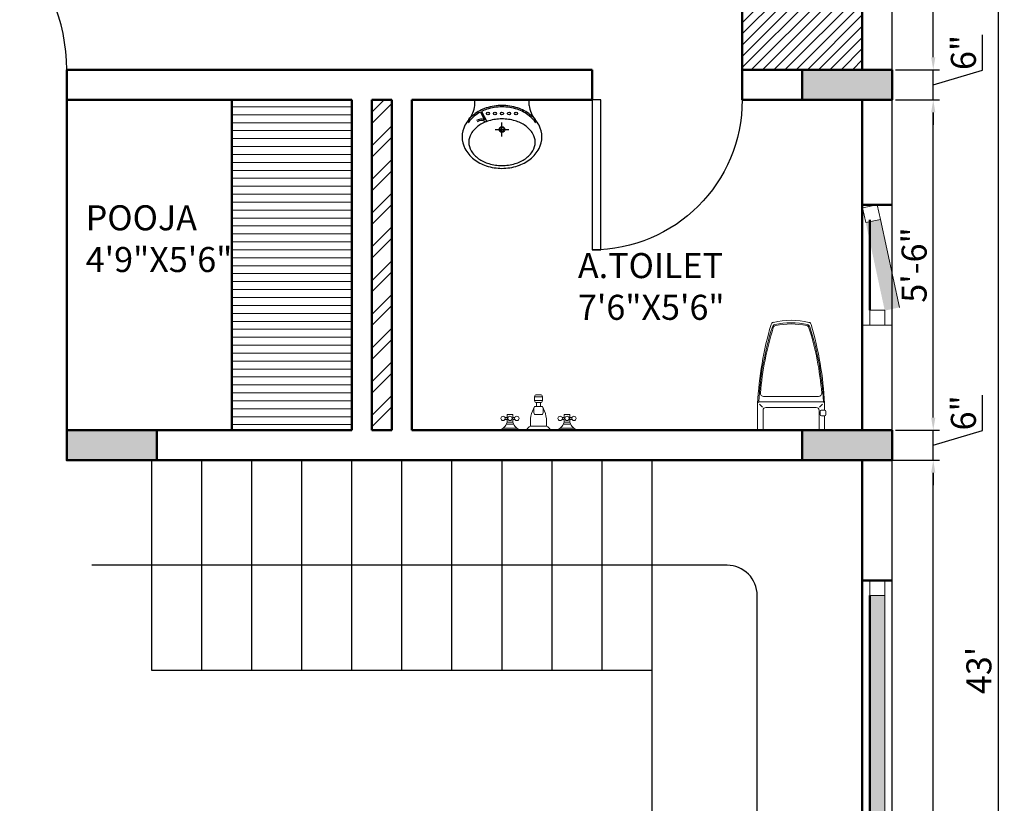
# Model space of a CAD drawing. Units: inches. Extents: x 3064 to 19385, y 846 to 15425.
# Tile 29 of 108: x 4932 to 5129, y 1108 to 1264. Entities that reach past the tile are written whole.
import ezdxf

# ---------------------------------------------------------------- set-up
doc = ezdxf.new("R2010")
doc.units = ezdxf.units.IN
for name, color, linetype, lineweight in [('A-ANNO-DIMS', 2, 'Continuous', 18), ('A-AREA-IDEN', 3, 'Continuous', 18), ('A-COLS', 1, 'Continuous', 35), ('A-DOOR', 3, 'Continuous', 25), ('A-FLOR-FIXT', 9, 'Continuous', 18), ('A-FLOR-STRS', 2, 'Continuous', 25), ('A-FURN-PATT', 252, 'Continuous', 13), ('A-GLAZ', 4, 'Continuous', 18), ('A-WALL', 7, 'Continuous', 50), ('C-PROP', 6, 'Continuous', 25)]:
    doc.layers.add(name, color=color, linetype=linetype, lineweight=lineweight)
doc.layers.add('THIET-BI', color=21, linetype='Continuous')
doc.styles.get("Standard").update_dxf_attribs({"font": 'arial.ttf'})
doc.dimstyles.new('ISO-25', dxfattribs={"dimtxt": 9, "dimasz": 2.5, "dimexe": 1.25, "dimexo": 0.625, "dimtad": 1, "dimdec": 1, "dimlunit": 3, "dimtxsty": 'Standard', "dimcen": 2.5, "dimadec": 0, "dimazin": 0, "dimtfac": 1, "dimtdec": 1, "dimtmove": 0, "dimatfit": 3, "dimfxl": 1, "dimarcsym": 0})

# ---------------------------------------------------------------- blocks, each defined once
blk = doc.blocks.new('*U3')
for p, q in [((0, 0), (0, -6)), ((36, 0), (36, -6))]:
    blk.add_line(p, q)
blk.add_lwpolyline([(0, 0), (0, 36), (1.75, 36), (1.75, 0)], close=True)
blk.add_arc((0, 0), 36, 0, 90)
blk = doc.blocks.new('*U4')
for p, q in [((0, 0), (0, -6)), ((30, 0), (30, -6))]:
    blk.add_line(p, q)
blk.add_lwpolyline([(0, 0), (0, 30), (1.75, 30), (1.75, 0)], close=True)
blk.add_arc((0, 0), 30, 0, 90)
blk = doc.blocks.new('A$C430D11A0')
at = {"layer": 'THIET-BI'}
for p, q in [((90, 445), (90, 485)), ((475, 485), (90, 485)), ((475, 483), (90, 483)), ((475, 445), (475, 485)), ((129.4, 398.5), (158.2, 344.4)), ((138.3, 403), (176, 332.4)), ((282.5, 226.2), (282.5, 324.8)), ((233.4, 275.5), (331.9, 275.5))]:
    blk.add_line(p, q, dxfattribs=at)
for points in [[(565, 222.5, 0.121635), (544.7, 304.8, 0.10526), (482.3, 379.8, 0.088175), (393.4, 427.4, 0.079002), (282.5, 445, 0.079002), (171.6, 427.4, 0.088175), (82.7, 379.8, 0.10526), (20.3, 304.8, 0.121635), (0, 222.5, 0.121635), (20.3, 140.2, 0.10526), (82.7, 65.2, 0.088175), (171.6, 17.6, 0.079002), (282.5, 0, 0.079002), (393.4, 17.6, 0.088175), (482.3, 65.2, 0.10526), (544.7, 140.2, 0.121635)], [(517.5, 185, 0.134042), (501.2, 244.9, 0.106817), (448.7, 301.7, 0.082468), (375.6, 336.7, 0.070874), (282.5, 350, 0.070874), (189.4, 336.7, 0.082468), (116.3, 301.7, 0.106817), (63.8, 244.9, 0.134042), (47.5, 185, 0.134042), (63.8, 125.1, 0.106817), (116.3, 68.3, 0.082468), (189.4, 33.3, 0.070874), (282.5, 20, 0.070874), (375.6, 33.3, 0.082468), (448.7, 68.3, 0.106817), (501.2, 125.1, 0.134042)]]:
    blk.add_lwpolyline(points, format="xyb", close=True, dxfattribs=at)
for points in [[(522.9, 321.6, 0.07708), (476.1, 372, 0.088175), (390.3, 417.9, 0.079002), (282.5, 435, 0.079002), (174.7, 417.9, 0.035427), (138.3, 403, 0.07708)], [(129.4, 398.5, 0.043566), (88.9, 372, 0.07708), (42.1, 321.6, 0.041486)]]:
    blk.add_lwpolyline(points, format="xyb", dxfattribs=at)
for centre, radius in [((182.5, 388.2), 10.5), ((232.5, 388.2), 10.5), ((282.5, 388.2), 10.5), ((332.5, 388.2), 10.5), ((382.5, 388.2), 10.5), ((282.5, 275.5), 20), ((282.5, 275.5), 15)]:
    blk.add_circle(centre, radius, dxfattribs=at)
for centre, radius, start, end in [((-103.8, 468.9), 195.3, 320.8253, 352.95569), ((668.8, 468.9), 195.3, 187.04431, 219.1747), ((136.4, 285.4), 62.9, 69.64296, 123.47738), ((136.4, 285.4), 52.9, 55.24551, 123.47738)]:
    blk.add_arc(centre, radius, start, end, dxfattribs=at)
blk = doc.blocks.new('WC-P05')
for p, q in [((-202.4, 531.6), (-202.4, 439.1)), ((-192.4, 541.6), (262.6, 541.6)), ((-163.4, 541.6), (-163.4, 400.6)), ((233.6, 541.6), (233.6, 400.6)), ((272.6, 531.6), (272.6, 351.6)), ((-210.4, 430.1), (-210.4, 409.1)), ((-201.4, 439.1), (-180.4, 439.1)), ((-171.4, 430.1), (-171.4, 409.1)), ((-202.4, 400.1), (-202.4, 351.6)), ((-201.4, 400.1), (-180.4, 400.1)), ((-166.9, 378.6), (-188.2, 357.3)), ((-143.4, 380.6), (213.6, 380.6)), ((237.1, 378.6), (258.4, 357.3)), ((-192.4, 341.6), (262.6, 341.6)), ((-159.3, 302.6), (229.5, 302.6))]:
    blk.add_line(p, q)
blk.add_lwpolyline([(-90.9, -221.9, 0.114547), (161, -222, 0.114547)], format="xyb")
for centre, radius, start, end in [((-192.4, 531.6), 10, 90, 180), ((262.6, 531.6), 10, 0, 90), ((-201.4, 430.1), 9, 90, 180), ((-180.4, 430.1), 9, 0, 90), ((-201.4, 409.1), 9, 180, 270), ((2308.9, 492.3), 2515.2, 183.20675, 196.12415), ((-192.4, 351.6), 10, 180, 270), ((-180.4, 409.1), 9, 270, 0), ((-143.4, 400.6), 20, 180, 270), ((-2238.7, 492.3), 2515.2, 343.87268, 356.79325), ((213.6, 400.6), 20, 270, 0), ((262.6, 351.6), 10, 270, 0), ((1906, 447.2), 2102.6, 182.87428, 197.65536), ((-159.3, 280.1), 22.5, 90, 184.62462), ((-1835.8, 447.2), 2102.6, 342.34464, 357.12572), ((229.5, 280.1), 22.5, 355.37538, 90), ((1905.9, 447.2), 2094.5, 184.62454, 197.52765), ((-1835.8, 447.2), 2094.6, 342.46396, 355.37538), ((-85.8, -199.9), 22.5, 196.12415, 256.89941), ((-76.1, -183.7), 22.5, 197.65536, 257.50587), ((-69.9, -176.8), 22.5, 197.52765, 258.10049), ((35.1, 318), 536.4, 257.50587, 282.49413), ((35.7, 324.3), 534.7, 258.10049, 281.73735), ((139.9, -177.1), 22.5, 281.73735, 342.46396), ((146.2, -183.7), 22.5, 282.49413, 342.34464), ((155.9, -200.1), 22.5, 283.03778, 343.87268)]:
    blk.add_arc(centre, radius, start, end)
blk = doc.blocks.new('Faucet - Bathroom front')
for p, q in [((-0.5, 4.25), (0.5, 4.25)), ((0.5, 3.75), (-0.5, 3.75)), ((-0.5, 3), (0.5, 3)), ((-0.25, 3), (-0.25, 3.5)), ((0.25, 3.5), (0.25, 3)), ((-4, 1.625), (-4.25, 1.625)), ((-4, 1.375), (-4.25, 1.375)), ((-3.25, 1.625), (-3, 1.625)), ((-3.25, 1.375), (-3, 1.375)), ((0.5, 2), (-0.5, 2)), ((3.25, 1.625), (3, 1.625)), ((3.25, 1.375), (3, 1.375)), ((4, 1.625), (4.25, 1.625)), ((4, 1.375), (4.25, 1.375)), ((-5, 0), (-2.25, 0)), ((-4.5087, 0.25), (-2.7408, 0.25)), ((-3.1442, 0.75), (-4.0979, 0.75)), ((-1.5, 0), (1.5, 0)), ((-1, 0.5), (1, 0.5)), ((2.25, 0), (5, 0)), ((2.7413, 0.25), (4.5092, 0.25)), ((4.1058, 0.75), (3.1521, 0.75))]:
    blk.add_line(p, q)
for points in [[(-0.5, 3.75), (-0.5, 4.25)], [(-0.25, 4.5), (0.25, 4.5)], [(0.5, 4.25), (0.5, 3.75)], [(0.25, 3.5), (-0.25, 3.5)]]:
    blk.add_lwpolyline(points)
for points in [[(-4, 1), (-4, 2), (-3.25, 2), (-3.25, 1)], [(3.25, 1), (3.25, 2), (4, 2), (4, 1)]]:
    blk.add_lwpolyline(points, close=True)
for centre in [(-4.5, 1.5), (-3.625, 1.5), (-2.75, 1.5), (2.75, 1.5), (3.625, 1.5), (4.5, 1.5)]:
    blk.add_circle(centre, 0.2795)
for centre, radius, start, end in [((-0.2575, 4.2575), 0.2426, 88.22243, 181.7776), ((0.2575, 4.2575), 0.2426, 358.2224, 91.77757), ((3, 1), 4.0311, 150.2551, 187.125), ((0.6413, 2.5), 1.246, 156.3417, 203.6583), ((-0.2575, 3.7425), 0.2426, 178.2224, 271.7776), ((0.2575, 3.7425), 0.2426, 268.2224, 1.777565), ((-3, 1), 4.0311, 352.875, 29.74488), ((-0.6413, 2.5), 1.246, 336.3417, 23.65835), ((-5.375, 1.375), 1.4252, 285.2551, 344.7449), ((-1.875, 1.375), 1.4252, 195.2551, 254.7449), ((-0.7962, -0.2038), 0.7327, 106.1502, 163.8498), ((0.7962, -0.2038), 0.7327, 16.1502, 73.84979), ((1.875, 1.375), 1.4252, 285.2551, 344.7449), ((5.375, 1.375), 1.4252, 195.2551, 254.7449)]:
    blk.add_arc(centre, radius, start, end)
blk = doc.blocks.new('*D60')
at = {"layer": 'A-ANNO-DIMS', "color": 0, "lineweight": -2, "transparency": 16777216}
for p, q in [((5101.1, 1176.1), (5115.92, 1176.1)), ((5114.67, 980.6), (5114.67, 1173.6)), ((5101.1, 978.1), (5115.92, 978.1))]:
    blk.add_line(p, q, dxfattribs=at)
at = {"layer": 'A-ANNO-DIMS', "color": 0, "transparency": 16777216}
for points in [[(5114.25, 1173.6), (5115.09, 1173.6), (5114.67, 1176.1)], [(5114.25, 980.6), (5115.09, 980.6), (5114.67, 978.1)]]:
    blk.add_solid(points, dxfattribs=at)
at = {"layer": 'Defpoints', "color": 0, "transparency": 16777216}
for p in [(5100.48, 1176.1), (5114.67, 1176.1), (5100.48, 978.1)]:
    blk.add_point(p, dxfattribs=at)
at = {"layer": 'A-ANNO-DIMS', "color": 0, "transparency": 16777216, "insert": (5111.49, 1077.1), "char_height": 5, "attachment_point": 5, "rotation": 90}
blk.add_mtext('16\'-6"', dxfattribs=at)
blk = doc.blocks.new('*D61')
at = {"layer": 'A-ANNO-DIMS', "color": 0, "lineweight": -2, "transparency": 16777216}
for p, q in [((5124.52, 1182.05), (5124.52, 1189.07)), ((5114.67, 1184.6), (5114.67, 1187.1)), ((5107.1, 1182.1), (5115.92, 1182.1)), ((5114.67, 1176.1), (5114.67, 1182.1)), ((5114.67, 1176.1), (5114.67, 1182.1)), ((5114.67, 1179.1), (5124.52, 1182.05)), ((5101.1, 1176.1), (5115.92, 1176.1)), ((5114.67, 1173.6), (5114.67, 1171.1))]:
    blk.add_line(p, q, dxfattribs=at)
at = {"layer": 'A-ANNO-DIMS', "color": 0, "transparency": 16777216}
for points in [[(5114.25, 1184.6), (5115.09, 1184.6), (5114.67, 1182.1)], [(5114.25, 1173.6), (5115.09, 1173.6), (5114.67, 1176.1)]]:
    blk.add_solid(points, dxfattribs=at)
at = {"layer": 'Defpoints', "color": 0, "transparency": 16777216}
for p in [(5106.48, 1182.1), (5114.67, 1182.1), (5100.48, 1176.1)]:
    blk.add_point(p, dxfattribs=at)
at = {"layer": 'A-ANNO-DIMS', "color": 0, "transparency": 16777216, "insert": (5121.34, 1185.56), "char_height": 5, "attachment_point": 5, "rotation": 90}
blk.add_mtext('6"', dxfattribs=at)
blk = doc.blocks.new('*D62')
at = {"layer": 'A-ANNO-DIMS', "color": 0, "lineweight": -2, "transparency": 16777216}
for p, q in [((5107.1, 1248.1), (5115.92, 1248.1)), ((5114.67, 1184.6), (5114.67, 1245.6)), ((5107.1, 1182.1), (5115.92, 1182.1))]:
    blk.add_line(p, q, dxfattribs=at)
at = {"layer": 'A-ANNO-DIMS', "color": 0, "transparency": 16777216}
for points in [[(5114.25, 1245.6), (5115.09, 1245.6), (5114.67, 1248.1)], [(5114.25, 1184.6), (5115.09, 1184.6), (5114.67, 1182.1)]]:
    blk.add_solid(points, dxfattribs=at)
at = {"layer": 'Defpoints', "color": 0, "transparency": 16777216}
for p in [(5106.48, 1248.1), (5114.67, 1248.1), (5106.48, 1182.1)]:
    blk.add_point(p, dxfattribs=at)
at = {"layer": 'A-ANNO-DIMS', "color": 0, "transparency": 16777216, "insert": (5111.49, 1215.1), "char_height": 5, "attachment_point": 5, "rotation": 90}
blk.add_mtext('5\'-6"', dxfattribs=at)
blk = doc.blocks.new('*D63')
at = {"layer": 'A-ANNO-DIMS', "color": 0, "lineweight": -2, "transparency": 16777216}
for p, q in [((5124.52, 1254.05), (5124.52, 1261.07)), ((5114.67, 1256.6), (5114.67, 1259.1)), ((5107.1, 1254.1), (5115.92, 1254.1)), ((5114.67, 1248.1), (5114.67, 1254.1)), ((5114.67, 1248.1), (5114.67, 1254.1)), ((5114.67, 1251.1), (5124.52, 1254.05)), ((5107.1, 1248.1), (5115.92, 1248.1)), ((5114.67, 1245.6), (5114.67, 1243.1))]:
    blk.add_line(p, q, dxfattribs=at)
at = {"layer": 'A-ANNO-DIMS', "color": 0, "transparency": 16777216}
for points in [[(5114.25, 1256.6), (5115.09, 1256.6), (5114.67, 1254.1)], [(5114.25, 1245.6), (5115.09, 1245.6), (5114.67, 1248.1)]]:
    blk.add_solid(points, dxfattribs=at)
at = {"layer": 'Defpoints', "color": 0, "transparency": 16777216}
for p in [(5106.48, 1254.1), (5114.67, 1254.1), (5106.48, 1248.1)]:
    blk.add_point(p, dxfattribs=at)
at = {"layer": 'A-ANNO-DIMS', "color": 0, "transparency": 16777216, "insert": (5121.34, 1257.56), "char_height": 5, "attachment_point": 5, "rotation": 90}
blk.add_mtext('6"', dxfattribs=at)
blk = doc.blocks.new('*D64')
at = {"layer": 'A-ANNO-DIMS', "color": 0, "lineweight": -2, "transparency": 16777216}
for p, q in [((5101.1, 1386.1), (5115.92, 1386.1)), ((5114.67, 1256.6), (5114.67, 1383.6)), ((5107.1, 1254.1), (5115.92, 1254.1))]:
    blk.add_line(p, q, dxfattribs=at)
at = {"layer": 'A-ANNO-DIMS', "color": 0, "transparency": 16777216}
for points in [[(5114.25, 1383.6), (5115.09, 1383.6), (5114.67, 1386.1)], [(5114.25, 1256.6), (5115.09, 1256.6), (5114.67, 1254.1)]]:
    blk.add_solid(points, dxfattribs=at)
at = {"layer": 'Defpoints', "color": 0, "transparency": 16777216}
for p in [(5100.48, 1386.1), (5114.67, 1386.1), (5106.48, 1254.1)]:
    blk.add_point(p, dxfattribs=at)
at = {"layer": 'A-ANNO-DIMS', "color": 0, "transparency": 16777216, "insert": (5111.53, 1320.1), "char_height": 5, "attachment_point": 5, "rotation": 90}
blk.add_mtext("11'", dxfattribs=at)
blk = doc.blocks.new('*D66')
at = {"layer": 'A-ANNO-DIMS', "color": 0, "lineweight": -2, "transparency": 16777216}
for p, q in [((5107.1, 1392.1), (5128.87, 1392.1)), ((5127.62, 1389.6), (5127.62, 878.6)), ((5107.1, 876.1), (5128.87, 876.1))]:
    blk.add_line(p, q, dxfattribs=at)
at = {"layer": 'A-ANNO-DIMS', "color": 0, "transparency": 16777216}
for points in [[(5127.2, 1389.6), (5128.04, 1389.6), (5127.62, 1392.1)], [(5127.2, 878.6), (5128.04, 878.6), (5127.62, 876.1)]]:
    blk.add_solid(points, dxfattribs=at)
at = {"layer": 'Defpoints', "color": 0, "transparency": 16777216}
for p in [(5106.48, 1392.1), (5106.48, 876.1), (5127.62, 876.1)]:
    blk.add_point(p, dxfattribs=at)
at = {"layer": 'A-ANNO-DIMS', "color": 0, "transparency": 16777216, "insert": (5124.44, 1134.1), "char_height": 5, "attachment_point": 5, "rotation": 90}
blk.add_mtext("43'", dxfattribs=at)
blk = doc.blocks.new('WIN-600')
h = blk.add_hatch(color=256)
h.dxf.hatch_style = 1
h.paths.add_polyline_path([(3, 18), (0, 18), (0, 0), (3, 0)])
blk.add_line((3, 18), (3, 0))
blk.add_lwpolyline([(3, 18), (0, 18), (0, 21), (3, 21)], close=True)
blk = doc.blocks.new('WIN-1800-PAIR')
h = blk.add_hatch(color=256)
h.dxf.hatch_style = 1
h.paths.add_polyline_path([(0, 0), (3, 0), (3, 70.5), (0, 70.5)])
h.paths.add_polyline_path([(3, 144), (0, 144), (0, 73.5), (3, 73.5)])
blk.add_line((3, 144), (3, 73.5))
blk.add_lwpolyline([(3, 144), (0, 144), (0, 147), (3, 147)], close=True)

msp = doc.modelspace()

# ---------------------------------------------------------------- hatches: boundary and pattern name
at = {"layer": 'A-COLS'}
h = msp.add_hatch(color=256, dxfattribs=at)
h.dxf.hatch_style = 1
h.paths.add_polyline_path([(5106.48, 1254.1), (5088.48, 1254.1), (5088.48, 1248.1), (5106.48, 1248.1)])
h = msp.add_hatch(color=256, dxfattribs=at)
h.dxf.hatch_style = 1
h.paths.add_polyline_path([(4959.48, 1182.1), (4941.48, 1182.1), (4941.48, 1176.1), (4959.48, 1176.1)])
h = msp.add_hatch(color=256, dxfattribs=at)
h.dxf.hatch_style = 1
h.paths.add_polyline_path([(5106.48, 1182.1), (5088.48, 1182.1), (5088.48, 1176.1), (5106.48, 1176.1)])
at = {"layer": 'A-FURN-PATT'}
h = msp.add_hatch(dxfattribs=at)
h.set_pattern_fill('ANSI31', color=256, scale=0.5)
h.set_pattern_definition([(45, (-551.1915, -4.2436), (-1.122532, 1.122532), [])])
h.paths.add_polyline_path([(5076.48, 1254.1), (5100.48, 1254.1), (5100.48, 1386.1), (5076.48, 1386.1)])
h = msp.add_hatch(dxfattribs=at)
h.set_pattern_fill('ANSI31', color=256, scale=0.5, angle=135)
h.set_pattern_definition([(180, (-551.1915, -4.2436), (-1e-16, -1.5875), [])])
h.paths.add_polyline_path([(4974.48, 1182.1), (4998.48, 1182.1), (4998.48, 1248.1), (4974.48, 1248.1)])
h = msp.add_hatch(dxfattribs=at)
h.set_pattern_fill('ANSI32', color=256, scale=0.5)
h.set_pattern_definition([(45, (-551.1915, -4.2436), (-3.367596, 3.367596), []), (45, (-548.9465, -4.2436), (-3.367596, 3.367596), [])])
h.paths.add_polyline_path([(5002.48, 1182.1), (5006.48, 1182.1), (5006.48, 1248.1), (5002.48, 1248.1)])

# ---------------------------------------------------------------- linework, layer by layer
at = {"layer": 'A-FLOR-STRS'}
for p, q in [((4958.48, 1134.1), (4958.48, 1176.1)), ((4968.48, 1134.1), (4968.48, 1176.1)), ((4978.48, 1134.1), (4978.48, 1176.1)), ((4988.48, 1134.1), (4988.48, 1176.1)), ((4998.48, 1134.1), (4998.48, 1176.1)), ((5008.48, 1134.1), (5008.48, 1176.1)), ((5018.48, 1134.1), (5018.48, 1176.1)), ((5028.48, 1134.1), (5028.48, 1176.1)), ((5038.48, 1134.1), (5038.48, 1176.1)), ((5048.48, 1134.1), (5048.48, 1176.1)), ((5058.48, 1020.1), (5058.48, 1176.1)), ((5058.48, 1134.1), (4958.48, 1134.1))]:
    msp.add_line(p, q, dxfattribs=at)
msp.add_lwpolyline([(4965.97, 999.1), (5073.48, 999.1, 0.414214), (5079.48, 1005.1), (5079.48, 1149.1, 0.414214), (5073.48, 1155.1), (4946.48, 1155.1)], format="xyb", dxfattribs=at)
at = {"layer": 'A-GLAZ'}
msp.add_line((5100.48, 1203.1), (5106.48, 1203.1), dxfattribs=at)
msp.add_lwpolyline([(5104.98, 1203.1), (5101.98, 1203.1), (5101.98, 1206.1), (5104.98, 1206.1)], close=True, dxfattribs=at)
at = {"layer": 'A-WALL'}
for p, q in [((5076.48, 1248.1), (5076.48, 1386.1)), ((5100.48, 1254.1), (5100.48, 1386.1)), ((5046.48, 1254.1), (4941.48, 1254.1)), ((4941.48, 1254.1), (4941.48, 1176.1)), ((5046.48, 1248.1), (5046.48, 1254.1)), ((5100.48, 1254.1), (5076.48, 1254.1)), ((4998.48, 1248.1), (4941.48, 1248.1)), ((4974.48, 1248.1), (4974.48, 1182.1)), ((4998.48, 1248.1), (4998.48, 1182.1)), ((5006.48, 1248.1), (5002.48, 1248.1)), ((5002.48, 1248.1), (5002.48, 1182.1)), ((5006.48, 1182.1), (5006.48, 1248.1)), ((5010.48, 1182.1), (5010.48, 1248.1)), ((5046.48, 1248.1), (5010.48, 1248.1)), ((5100.48, 1248.1), (5076.48, 1248.1)), ((5100.48, 1182.1), (5100.48, 1248.1)), ((5100.48, 1227.1), (5106.48, 1227.1)), ((5101.98, 1224.1), (5101.98, 1206.1)), ((4998.48, 1182.1), (4941.48, 1182.1)), ((5006.48, 1182.1), (5002.48, 1182.1)), ((5100.48, 1182.1), (5010.48, 1182.1)), ((5100.48, 1176.1), (4941.48, 1176.1)), ((5100.48, 978.1), (5100.48, 1176.1)), ((5106.48, 1152.1), (5100.48, 1152.1)), ((5101.98, 1149.1), (5101.98, 1078.6))]:
    msp.add_line(p, q, dxfattribs=at)
for points in [[(5106.48, 1254.1), (5088.48, 1254.1), (5088.48, 1248.1), (5106.48, 1248.1)], [(4959.48, 1182.1), (4941.48, 1182.1), (4941.48, 1176.1), (4959.48, 1176.1)], [(5106.48, 1182.1), (5088.48, 1182.1), (5088.48, 1176.1), (5106.48, 1176.1)]]:
    msp.add_lwpolyline(points, close=True, dxfattribs=at)
at = {"layer": 'C-PROP'}
msp.add_line((5106.48, 876.1), (5106.48, 1392.1), dxfattribs=at)

# ---------------------------------------------------------------- block references
at = {"layer": 'A-DOOR'}
msp.add_blockref('*U3', (4905.48, 1254.1), dxfattribs=at)
at = {"layer": 'A-DOOR', "xscale": -1, "rotation": 180}
msp.add_blockref('*U4', (5046.48, 1248.1), dxfattribs=at)
at = {"layer": 'A-FLOR-FIXT'}
for name, p, xscale, yscale, zscale in [('A$C430D11A0', (5020.5, 1234.41), 0.0282220760332506, 0.0282220760332506, 0.0282220760332506), ('Faucet - Bathroom front', (5035.77, 1182.1), 1.573166238287219, 1.573166238287219, 1.573166238287219)]:
    msp.add_blockref(name, p, dxfattribs=dict(at, xscale=xscale, yscale=yscale, zscale=zscale))
at = {"layer": 'A-FLOR-FIXT', "xscale": 0.0282220760332506, "yscale": 0.0282220760332506, "zscale": 0.0282220760332506, "rotation": 180}
msp.add_blockref('WC-P05', (5087.25, 1197.38), dxfattribs=at)
at = {"layer": 'A-GLAZ', "rotation": 12.21571913413076}
msp.add_blockref('WIN-600', (5104.98, 1205.99), dxfattribs=at)
at = {"layer": 'A-GLAZ'}
msp.add_blockref('WIN-1800-PAIR', (5101.98, 1005.1), dxfattribs=at)

# ---------------------------------------------------------------- texts
at = {"layer": 'A-AREA-IDEN', "char_height": 5, "attachment_point": 1}
for s, insert in [('POOJA\\P4\'9"X5\'6"', (4945.27, 1227.03)), ('A.TOILET\\P7\'6"X5\'6"', (5043.65, 1217.48))]:
    msp.add_mtext_dynamic_manual_height_columns(s, width=67.5924, gutter_width=12.5, heights=[0], dxfattribs=dict(at, insert=insert))

# ---------------------------------------------------------------- dimensions: what is measured, and where the dimension line sits
at = {"layer": 'A-ANNO-DIMS'}
for base, p1, p2, override, picture, middle in [((5127.62, 876.1), (5106.48, 1392.1), (5106.48, 876.1), {"dimtxt": 5, "dimclrd": 0, "dimclre": 0, "dimclrt": 0}, '*D66', (5124.44, 1134.1)), ((5114.67, 1386.1), (5106.48, 1254.1), (5100.48, 1386.1), {"dimtxt": 5, "dimclrd": 0, "dimclre": 0, "dimclrt": 0, "dimtmove": 1}, '*D64', (5111.53, 1320.1)), ((5114.67, 1254.1), (5106.48, 1248.1), (5106.48, 1254.1), {"dimtxt": 5, "dimclrd": 0, "dimclre": 0, "dimclrt": 0, "dimtmove": 1}, '*D63', (5121.34, 1254.68)), ((5114.67, 1248.1), (5106.48, 1182.1), (5106.48, 1248.1), {"dimtxt": 5, "dimclrd": 0, "dimclre": 0, "dimclrt": 0, "dimtmove": 1}, '*D62', (5111.49, 1215.1)), ((5114.67, 1182.1), (5100.48, 1176.1), (5106.48, 1182.1), {"dimtxt": 5, "dimclrd": 0, "dimclre": 0, "dimclrt": 0, "dimtmove": 1}, '*D61', (5121.34, 1182.68)), ((5114.67, 1176.1), (5100.48, 978.1), (5100.48, 1176.1), {"dimtxt": 5, "dimclrd": 0, "dimclre": 0, "dimclrt": 0, "dimtmove": 1}, '*D60', (5111.49, 1077.1))]:
    dim = msp.add_linear_dim(base=base, p1=p1, p2=p2, angle=90, dimstyle='ISO-25', override=override, dxfattribs=at)
    dim.commit()
    dim.dimension.update_dxf_attribs({"geometry": picture, "text_midpoint": middle})

doc.saveas('drawing.dxf')
